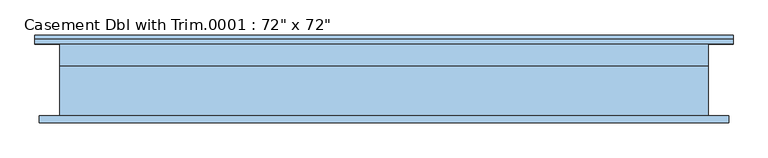
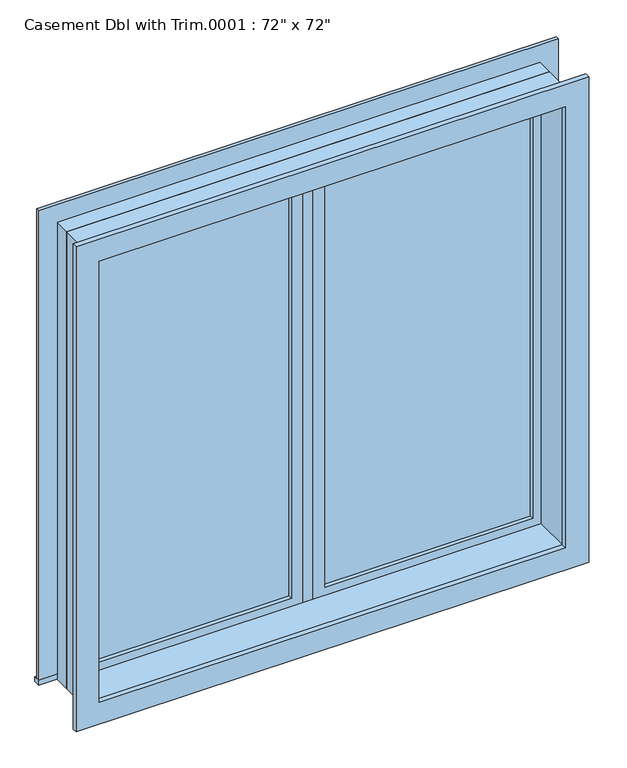
"""IFC4 building model written with IfcOpenShell, lengths in millimetres: window geometry."""

from ifc_helpers import new_model, si_unit, frame, origin, place, context, project, spatial, polyline, outline, extrude, source, transform, mapped, element, save


def window_97c6202a(model_context):
    return source(origin(), model_context, "Body", "SweptSolid", [
        extrude(outline(polyline([(63.5, 85.725), (850.9, 85.725), (850.9, 73.025), (63.5, 73.025), (63.5, 85.725)])), frame((0.0, 0.0, 977.9), z_axis=(0.0, 0.0, 1.0), x_axis=(1.0, 0.0, 0.0)), (0.0, 0.0, 1.0), 1701.8),
        extrude(outline(polyline([(2724.15, 19.05), (933.45, 19.05), (933.45, 895.35), (2724.15, 895.35), (2724.15, 19.05)]), holes=[polyline([(2679.7, 63.5), (2679.7, 850.9), (977.9, 850.9), (977.9, 63.5), (2679.7, 63.5)])]), frame((0.0, 57.15, 0.0), z_axis=(0.0, 1.0, 0.0), x_axis=(0.0, 0.0, 1.0)), (0.0, 0.0, 1.0), 44.45),
        extrude(outline(polyline([(19.05, 57.15), (-19.05, 57.15), (-19.05, 120.65), (19.05, 120.65), (19.05, 57.15)])), frame((0.0, 0.0, 933.45), z_axis=(0.0, 0.0, 1.0), x_axis=(1.0, 0.0, 0.0)), (0.0, 0.0, 1.0), 1790.7),
        extrude(outline(polyline([(-984.25, 146.05), (984.25, 146.05), (984.25, 120.65), (-984.25, 120.65), (-984.25, 146.05)])), frame((0.0, 0.0, 914.4), z_axis=(0.0, 0.0, 1.0), x_axis=(1.0, 0.0, 0.0)), (0.0, 0.0, 1.0), 19.05),
        extrude(outline(polyline([(2724.15, -895.35), (2724.15, 895.35), (933.45, 895.35), (933.45, 984.25), (2813.05, 984.25), (2813.05, -984.25), (933.45, -984.25), (933.45, -895.35), (2724.15, -895.35)])), frame((0.0, 120.65, 0.0), z_axis=(0.0, 1.0, 0.0), x_axis=(0.0, 0.0, 1.0)), (0.0, 0.0, 1.0), 12.7),
        extrude(outline(polyline([(2800.35, 971.55), (2800.35, -971.55), (857.25, -971.55), (857.25, 971.55), (2800.35, 971.55)]), holes=[polyline([(2711.45, 882.65), (946.15, 882.65), (946.15, -882.65), (2711.45, -882.65), (2711.45, 882.65)])]), frame((0.0, -101.6, 0.0), z_axis=(0.0, 1.0, 0.0), x_axis=(0.0, 0.0, 1.0)), (0.0, 0.0, 1.0), 19.05),
        extrude(outline(polyline([(-63.5, 73.025), (-850.9, 73.025), (-850.9, 85.725), (-63.5, 85.725), (-63.5, 73.025)])), frame((0.0, 0.0, 977.9), z_axis=(0.0, 0.0, 1.0), x_axis=(1.0, 0.0, 0.0)), (0.0, 0.0, 1.0), 1701.8),
        extrude(outline(polyline([(2724.15, -895.35), (933.45, -895.35), (933.45, -19.05), (2724.15, -19.05), (2724.15, -895.35)]), holes=[polyline([(2679.7, -850.9), (2679.7, -63.5), (977.9, -63.5), (977.9, -850.9), (2679.7, -850.9)])]), frame((0.0, 57.15, 0.0), z_axis=(0.0, 1.0, 0.0), x_axis=(0.0, 0.0, 1.0)), (0.0, 0.0, 1.0), 44.45),
        extrude(outline(polyline([(2743.2, -914.4), (914.4, -914.4), (914.4, 914.4), (2743.2, 914.4), (2743.2, -914.4)]), holes=[polyline([(2711.45, -882.65), (2711.45, 882.65), (946.15, 882.65), (946.15, -882.65), (2711.45, -882.65)])]), frame((0.0, -82.55, 0.0), z_axis=(0.0, 1.0, 0.0), x_axis=(0.0, 0.0, 1.0)), (0.0, 0.0, 1.0), 139.7),
        extrude(outline(polyline([(2743.2, 914.4), (2743.2, -914.4), (914.4, -914.4), (914.4, 914.4), (2743.2, 914.4)]), holes=[polyline([(2724.15, 895.35), (933.45, 895.35), (933.45, -895.35), (2724.15, -895.35), (2724.15, 895.35)])]), frame((0.0, 57.15, 0.0), z_axis=(0.0, 1.0, 0.0), x_axis=(0.0, 0.0, 1.0)), (0.0, 0.0, 1.0), 63.5),
    ])


if __name__ == "__main__":
    model = new_model("IFC4")
    model_context = context("Model", 3, world=origin())
    ifc_project = project(units=[si_unit("LENGTHUNIT", "METRE", prefix="MILLI")], contexts=[model_context])
    site = spatial("IfcSite", under=ifc_project)
    building = spatial("IfcBuilding", under=site)
    placement = place(None, origin())
    window_shape = window_97c6202a(model_context)
    element("IfcWindow", 1, ObjectType="Casement Dbl with Trim.0001 : 72\" x 72\"", at=placement, inside=building, context=model_context, shape_type="MappedRepresentation", body=[
        mapped(window_shape, transform((0.0, 0.0, 0.0), x_axis=(1.0, 0.0, 0.0), y_axis=(0.0, 1.0, 0.0), z_axis=(0.0, 0.0, 1.0))),
    ])
    save(model, "model.ifc")

# Revit data of these elements
# Type "Casement Dbl with Trim.0001 : 72\" x 72\""
#   Type Mark = "10"
#   Construction Type Id = "GSP4R"
#   Assembly Code = "B2020100"
#   Analytic Construction = "1/8 in Pilkington single glazing"
#   Visual Light Transmittance = 0.9
#   Solar Heat Gain Coefficient = 0.78
#   Heat Transfer Coefficient (U) = 0.6496 BTU/(h·ft²·°F)
#   Height = 6' - 0"
#   Default Sill Height = 3' - 0"
#   Trim Projection - Ext. = 0' - 0 1/2"
#   Trim Projection - Int. = 0' - 0 3/4"
#   Trim Width - Exterior = 0' - 3 1/2"
#   Trim Width - Interior = 0' - 3 1/2"
#   Width = 6' - 0"
#   Window Inset = 0' - 0 3/4"
#   Define Thermal Properties by = 1
#   Glass Pane Material = Glass
#   Sash Material = Iron, Ductile
#   Trim Exterior Material = Iron, Ductile
#   Trim Interior Material = Iron, Ductile
#   Wall Closure = (empty or 0)
# Element 1 (IfcWindow, "Casement Dbl with Trim.0001 : 72\" x 72\"")
#   Materials on its faces: "Iron, Ductile", "Glass"
# Materials
#   "Glass": class "Glass", colour RGB 0 128 192, transparency 0.75, Description = "Soda Lime Glass", Cost = 0
#   "Iron, Ductile": class "Metal", colour RGB 0 0 0, transparency 0, Description = "Ductile cast iron", Cost = 0
